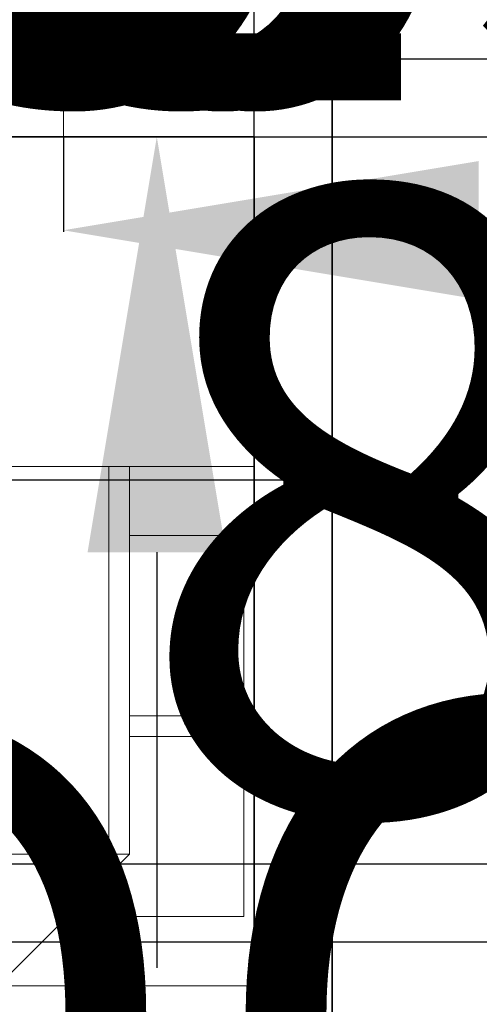
# Model space of a CAD drawing. Units: inches. Extents: x -307 to 2141, y -58 to 895.
# Tile 24 of 28: x 880 to 933, y 582 to 696. Entities that reach past the tile are written whole.
import ezdxf

# ---------------------------------------------------------------- set-up
doc = ezdxf.new("R2010")
doc.units = ezdxf.units.IN
doc.header["$MEASUREMENT"] = 0
for name, color, linetype, lineweight in [('A-ANNO-DIMS', 2, 'Continuous', 18), ('A-FURN', 8, 'Continuous', 18), ('A-GLAZ', 4, 'Continuous', 18), ('A-WALL', 7, 'Continuous', 35)]:
    doc.layers.add(name, color=color, linetype=linetype, lineweight=lineweight)
doc.styles.get("Standard").update_dxf_attribs({"font": 'arial.ttf'})
doc.dimstyles.get("Standard").update_dxf_attribs({"dimtxt": 72, "dimasz": 48, "dimexe": 0.18, "dimexo": 0.0625, "dimgap": 0.09, "dimtad": 0, "dimtih": 1, "dimtoh": 1, "dimdec": 0, "dimrnd": 48, "dimzin": 0, "dimdsep": 46, "dimlunit": 3, "dimtxsty": 'Standard', "dimcen": 0.09, "dimadec": 0, "dimazin": 0, "dimtfac": 1, "dimtdec": 0, "dimtofl": 0, "dimtmove": 0, "dimatfit": 3, "dimfxl": 1, "dimtolj": 1, "dimtzin": 0, "dimarcsym": 0})

# ---------------------------------------------------------------- blocks, each defined once
blk = doc.blocks.new('Bed - Queen')
for p, q in [((0, -80.00003), (0, 0)), ((0, 0), (59.99999, 0)), ((59.99999, 0), (59.99999, -80.00003)), ((7.99999, -1.2), (28.79998, -1.2)), ((7.99999, -14.4), (7.99999, -1.2)), ((28.79998, -1.2), (28.79998, -14.4)), ((31.19999, -1.2), (51.99999, -1.2)), ((31.19999, -14.4), (31.19999, -1.2)), ((51.99999, -1.2), (51.99999, -16.4)), ((0, -14.4), (44.8, -14.4)), ((59.99999, -29.6), (44.8, -14.4)), ((44.8, -14.4), (44.8, -29.6)), ((44.8, -16.8), (0, -16.8)), ((51.99999, -16.4), (46.79936, -16.4)), ((44.8, -29.6), (59.99999, -29.6)), ((59.99999, -80.00003), (0, -80.00003))]:
    blk.add_line(p, q)
blk = doc.blocks.new('WIN-72IN')
blk.add_line((72, 4.5), (0, 4.5))
blk.add_lwpolyline([(72, 0), (0, 0), (0, 9), (72, 9)], close=True)
blk = doc.blocks.new('*D30')
at = {"layer": 'A-ANNO-DIMS', "color": 0, "lineweight": -2, "transparency": 16777216}
for p, q in [((570.74, 532.83), (570.74, 580.83)), ((570.74, 580.83), (618.74, 580.83)), ((565.4, 484.83), (570.92, 484.83)), ((565.4, 448.83), (570.92, 448.83)), ((570.74, 400.83), (570.74, 352.83))]:
    blk.add_line(p, q, dxfattribs=at)
at = {"layer": 'A-ANNO-DIMS', "color": 0, "transparency": 16777216}
for points in [[(562.74, 532.83), (578.74, 532.83), (570.74, 484.83)], [(562.74, 400.83), (578.74, 400.83), (570.74, 448.83)]]:
    blk.add_solid(points, dxfattribs=at)
at = {"layer": 'Defpoints', "color": 0, "transparency": 16777216}
for p in [(565.34, 484.83), (570.74, 484.83), (565.34, 448.83)]:
    blk.add_point(p, dxfattribs=at)
at = {"layer": 'A-ANNO-DIMS', "color": 0, "transparency": 16777216, "insert": (1030.17, 580.83), "char_height": 72, "attachment_point": 5}
blk.add_mtext('\\A1;WINDOW 36 TYP.', dxfattribs=at)
blk = doc.blocks.new('*D32')
at = {"layer": 'A-ANNO-DIMS', "color": 0, "lineweight": -2, "transparency": 16777216}
for p, q in [((813.29, 682.28), (813.29, 671.36)), ((885.29, 682.28), (885.29, 671.36)), ((765.29, 671.54), (717.29, 671.54)), ((933.29, 671.54), (981.29, 671.54))]:
    blk.add_line(p, q, dxfattribs=at)
at = {"layer": 'A-ANNO-DIMS', "color": 0, "transparency": 16777216}
for points in [[(765.29, 679.54), (765.29, 663.54), (813.29, 671.54)], [(933.29, 679.54), (933.29, 663.54), (885.29, 671.54)]]:
    blk.add_solid(points, dxfattribs=at)
at = {"layer": 'Defpoints', "color": 0, "transparency": 16777216}
for p in [(813.29, 682.34), (885.29, 682.34), (885.29, 671.54)]:
    blk.add_point(p, dxfattribs=at)
at = {"layer": 'A-ANNO-DIMS', "color": 0, "transparency": 16777216, "insert": (1392.73, 671.54), "char_height": 72, "attachment_point": 5}
blk.add_mtext('\\A1;WINDOW 72 TYP.', dxfattribs=at)
blk = doc.blocks.new('*D33')
at = {"layer": 'A-ANNO-DIMS', "color": 0, "lineweight": -2, "transparency": 16777216}
for p, q in [((896.09, 739.34), (896.09, 787.34)), ((896.09, 787.34), (944.09, 787.34)), ((885.36, 691.34), (896.27, 691.34)), ((885.36, 682.34), (896.27, 682.34)), ((896.09, 634.34), (896.09, 586.34))]:
    blk.add_line(p, q, dxfattribs=at)
at = {"layer": 'A-ANNO-DIMS', "color": 0, "transparency": 16777216}
for points in [[(888.09, 739.34), (904.09, 739.34), (896.09, 691.34)], [(888.09, 634.34), (904.09, 634.34), (896.09, 682.34)]]:
    blk.add_solid(points, dxfattribs=at)
at = {"layer": 'Defpoints', "color": 0, "transparency": 16777216}
for p in [(885.29, 691.34), (896.09, 691.34), (885.29, 682.34)]:
    blk.add_point(p, dxfattribs=at)
at = {"layer": 'A-ANNO-DIMS', "color": 0, "transparency": 16777216, "insert": (1091.45, 787.34), "char_height": 72, "attachment_point": 5}
blk.add_mtext('\\A1;9 TYP.', dxfattribs=at)
blk = doc.blocks.new('*D34')
at = {"layer": 'A-ANNO-DIMS', "color": 0, "lineweight": -2, "transparency": 16777216}
for p, q in [((927.14, 490.97), (927.14, 538.97)), ((927.14, 538.97), (975.14, 538.97)), ((916.4, 442.97), (927.32, 442.97)), ((916.4, 370.95), (927.32, 370.95)), ((927.14, 322.95), (927.14, 274.95))]:
    blk.add_line(p, q, dxfattribs=at)
at = {"layer": 'A-ANNO-DIMS', "color": 0, "transparency": 16777216}
for points in [[(919.14, 490.97), (935.14, 490.97), (927.14, 442.97)], [(919.14, 322.95), (935.14, 322.95), (927.14, 370.95)]]:
    blk.add_solid(points, dxfattribs=at)
at = {"layer": 'Defpoints', "color": 0, "transparency": 16777216}
for p in [(916.34, 442.97), (927.14, 442.97), (916.34, 370.95)]:
    blk.add_point(p, dxfattribs=at)
at = {"layer": 'A-ANNO-DIMS', "color": 0, "transparency": 16777216, "insert": (1584.53, 538.97), "char_height": 72, "attachment_point": 5}
blk.add_mtext('\\A1;PAIRED WINDOW 72 TYP.', dxfattribs=at)
blk = doc.blocks.new('*D37')
at = {"layer": 'A-ANNO-DIMS', "color": 0, "lineweight": -2, "transparency": 16777216}
for p, q in [((828.62, 519.41), (780.62, 519.46)), ((876.61, 514.46), (876.62, 519.54)), ((897.61, 514.44), (897.62, 519.51)), ((945.62, 519.28), (993.62, 519.22))]:
    blk.add_line(p, q, dxfattribs=at)
at = {"layer": 'A-ANNO-DIMS', "color": 0, "transparency": 16777216}
for points in [[(828.63, 527.41), (828.61, 511.41), (876.62, 519.36)], [(945.63, 527.28), (945.61, 511.28), (897.62, 519.33)]]:
    blk.add_solid(points, dxfattribs=at)
at = {"layer": 'Defpoints', "color": 0, "transparency": 16777216}
for p in [(876.62, 519.36), (876.61, 514.4), (897.61, 514.38)]:
    blk.add_point(p, dxfattribs=at)
at = {"layer": 'A-ANNO-DIMS', "color": 0, "transparency": 16777216, "insert": (604.68, 519.46), "char_height": 72, "attachment_point": 5}
blk.add_mtext('\\A1;21 TYP.', dxfattribs=at)
blk = doc.blocks.new('*D42')
at = {"layer": 'A-ANNO-DIMS', "color": 0, "lineweight": -2, "transparency": 16777216}
for p, q in [((880.26, 543.86), (928.25, 544.87)), ((822.3, 541.2), (822.27, 542.82)), ((832.3, 541.41), (832.27, 543.03)), ((774.28, 541.63), (726.29, 540.62))]:
    blk.add_line(p, q, dxfattribs=at)
at = {"layer": 'A-ANNO-DIMS', "color": 0, "transparency": 16777216}
for points in [[(880.09, 551.86), (880.43, 535.86), (832.27, 542.85)], [(774.11, 549.63), (774.45, 533.63), (822.27, 542.64)]]:
    blk.add_solid(points, dxfattribs=at)
at = {"layer": 'Defpoints', "color": 0, "transparency": 16777216}
for p in [(832.27, 542.85), (822.3, 541.14), (832.3, 541.35)]:
    blk.add_point(p, dxfattribs=at)
at = {"layer": 'A-ANNO-DIMS', "color": 0, "transparency": 16777216, "insert": (1192.89, 544.87), "char_height": 72, "attachment_point": 5}
blk.add_mtext('\\A1;FAUCET 10', dxfattribs=at)
blk = doc.blocks.new('*D44')
at = {"layer": 'A-ANNO-DIMS', "color": 0, "lineweight": -2, "transparency": 16777216}
for p, q in [((839.87, 521.22), (839.95, 517.42)), ((815.33, 520.71), (815.41, 516.91)), ((887.94, 518.61), (935.93, 519.62)), ((767.41, 516.08), (719.42, 515.07))]:
    blk.add_line(p, q, dxfattribs=at)
at = {"layer": 'A-ANNO-DIMS', "color": 0, "transparency": 16777216}
for points in [[(887.77, 526.61), (888.11, 510.61), (839.95, 517.6)], [(767.25, 524.08), (767.58, 508.08), (815.4, 517.09)]]:
    blk.add_solid(points, dxfattribs=at)
at = {"layer": 'Defpoints', "color": 0, "transparency": 16777216}
for p in [(839.87, 521.29), (815.33, 520.77), (839.95, 517.6)]:
    blk.add_point(p, dxfattribs=at)
at = {"layer": 'A-ANNO-DIMS', "color": 0, "transparency": 16777216, "insert": (1151.16, 519.62), "char_height": 72, "attachment_point": 5}
blk.add_mtext('\\A1;BASIN 25', dxfattribs=at)
blk = doc.blocks.new('*D46')
at = {"layer": 'A-ANNO-DIMS', "color": 0, "lineweight": -2, "transparency": 16777216}
for p, q in [((801.41, 645.78), (801.41, 642.52)), ((822.41, 645.78), (822.41, 642.52)), ((753.41, 642.7), (705.41, 642.7)), ((870.41, 642.7), (918.41, 642.7))]:
    blk.add_line(p, q, dxfattribs=at)
at = {"layer": 'A-ANNO-DIMS', "color": 0, "transparency": 16777216}
for points in [[(753.41, 650.7), (753.41, 634.7), (801.41, 642.7)], [(870.41, 650.7), (870.41, 634.7), (822.41, 642.7)]]:
    blk.add_solid(points, dxfattribs=at)
at = {"layer": 'Defpoints', "color": 0, "transparency": 16777216}
for p in [(801.41, 645.85), (822.41, 645.85), (822.41, 642.7)]:
    blk.add_point(p, dxfattribs=at)
at = {"layer": 'A-ANNO-DIMS', "color": 0, "transparency": 16777216, "insert": (1282.7, 642.7), "char_height": 72, "attachment_point": 5}
blk.add_mtext('\\A1;DESK CHAIR 21', dxfattribs=at)
blk = doc.blocks.new('*D47')
at = {"layer": 'A-ANNO-DIMS', "color": 0, "lineweight": -2, "transparency": 16777216}
for p, q in [((825.56, 711.18), (825.56, 759.18)), ((825.56, 759.18), (873.56, 759.18)), ((822.48, 663.18), (825.74, 663.18)), ((822.48, 645.85), (825.74, 645.85)), ((825.56, 597.85), (825.56, 549.85))]:
    blk.add_line(p, q, dxfattribs=at)
at = {"layer": 'A-ANNO-DIMS', "color": 0, "transparency": 16777216}
for points in [[(817.56, 711.18), (833.56, 711.18), (825.56, 663.18)], [(817.56, 597.85), (833.56, 597.85), (825.56, 645.85)]]:
    blk.add_solid(points, dxfattribs=at)
at = {"layer": 'Defpoints', "color": 0, "transparency": 16777216}
for p in [(822.41, 663.18), (825.56, 663.18), (822.41, 645.85)]:
    blk.add_point(p, dxfattribs=at)
at = {"layer": 'A-ANNO-DIMS', "color": 0, "transparency": 16777216, "insert": (921.83, 759.18), "char_height": 72, "attachment_point": 5}
blk.add_mtext('\\A1;17', dxfattribs=at)
blk = doc.blocks.new('*D52')
at = {"layer": 'A-ANNO-DIMS', "color": 0, "lineweight": -2, "transparency": 16777216}
for p, q in [((660.21, 554.25), (660.21, 602.25)), ((673.8, 506.25), (660.03, 506.25)), ((673.8, 415.25), (660.03, 415.25)), ((660.21, 367.25), (660.21, 319.25))]:
    blk.add_line(p, q, dxfattribs=at)
at = {"layer": 'A-ANNO-DIMS', "color": 0, "transparency": 16777216}
for points in [[(652.21, 554.25), (668.21, 554.25), (660.21, 506.25)], [(652.21, 367.25), (668.21, 367.25), (660.21, 415.25)]]:
    blk.add_solid(points, dxfattribs=at)
at = {"layer": 'Defpoints', "color": 0, "transparency": 16777216}
for p in [(673.86, 506.25), (660.21, 415.25), (673.86, 415.25)]:
    blk.add_point(p, dxfattribs=at)
at = {"layer": 'A-ANNO-DIMS', "color": 0, "transparency": 16777216, "insert": (660.21, 460.75), "char_height": 72, "attachment_point": 5}
blk.add_mtext('\\A1;DINING SET 91', dxfattribs=at)
blk = doc.blocks.new('*D56')
at = {"layer": 'A-ANNO-DIMS', "color": 0, "lineweight": -2, "transparency": 16777216}
for p, q in [((679.73, 723.21), (679.73, 771.21)), ((679.73, 771.21), (727.73, 771.21)), ((675.74, 675.21), (679.91, 675.21)), ((675.74, 648.21), (679.91, 648.21)), ((679.73, 600.21), (679.73, 552.21))]:
    blk.add_line(p, q, dxfattribs=at)
at = {"layer": 'A-ANNO-DIMS', "color": 0, "transparency": 16777216}
for points in [[(671.73, 723.21), (687.73, 723.21), (679.73, 675.21)], [(671.73, 600.21), (687.73, 600.21), (679.73, 648.21)]]:
    blk.add_solid(points, dxfattribs=at)
at = {"layer": 'Defpoints', "color": 0, "transparency": 16777216}
for p in [(675.68, 675.21), (679.73, 675.21), (675.68, 648.21)]:
    blk.add_point(p, dxfattribs=at)
at = {"layer": 'A-ANNO-DIMS', "color": 0, "transparency": 16777216, "insert": (1006.66, 771.21), "char_height": 72, "attachment_point": 5}
blk.add_mtext('\\A1;ROCKER 27', dxfattribs=at)
blk = doc.blocks.new('*D62')
at = {"layer": 'A-ANNO-DIMS', "color": 0, "lineweight": -2, "transparency": 16777216}
for p, q in [((556.34, 691.4), (556.34, 722.72)), ((604.34, 722.54), (656.85, 722.54)), ((868.34, 722.54), (815.82, 722.54)), ((916.34, 490.97), (916.34, 722.72))]:
    blk.add_line(p, q, dxfattribs=at)
at = {"layer": 'A-ANNO-DIMS', "color": 0, "transparency": 16777216}
for points in [[(604.34, 730.54), (604.34, 714.54), (556.34, 722.54)], [(868.34, 730.54), (868.34, 714.54), (916.34, 722.54)]]:
    blk.add_solid(points, dxfattribs=at)
at = {"layer": 'Defpoints', "color": 0, "transparency": 16777216}
for p in [(916.34, 722.54), (556.34, 691.34), (916.34, 490.9)]:
    blk.add_point(p, dxfattribs=at)
at = {"layer": 'A-ANNO-DIMS', "color": 0, "transparency": 16777216, "insert": (736.34, 722.54), "char_height": 72, "attachment_point": 5}
blk.add_mtext('\\A1;360', dxfattribs=at)
blk = doc.blocks.new('*D63')
at = {"layer": 'A-ANNO-DIMS', "color": 0, "lineweight": -2, "transparency": 16777216}
for p, q in [((916.4, 691.34), (947.72, 691.34)), ((947.54, 643.34), (947.54, 416.19)), ((947.54, 115.34), (947.54, 342.49)), ((704.68, 67.34), (947.72, 67.34))]:
    blk.add_line(p, q, dxfattribs=at)
at = {"layer": 'A-ANNO-DIMS', "color": 0, "transparency": 16777216}
for points in [[(939.54, 643.34), (955.54, 643.34), (947.54, 691.34)], [(939.54, 115.34), (955.54, 115.34), (947.54, 67.34)]]:
    blk.add_solid(points, dxfattribs=at)
at = {"layer": 'Defpoints', "color": 0, "transparency": 16777216}
for p in [(916.34, 691.34), (704.62, 67.34), (947.54, 67.34)]:
    blk.add_point(p, dxfattribs=at)
at = {"layer": 'A-ANNO-DIMS', "color": 0, "transparency": 16777216, "insert": (947.54, 379.34), "char_height": 72, "attachment_point": 5}
blk.add_mtext('\\A1;624', dxfattribs=at)
blk = doc.blocks.new('*D75')
at = {"layer": 'A-ANNO-DIMS', "color": 0, "lineweight": -2, "transparency": 16777216}
for p, q in [((565.34, 682.4), (565.34, 722.72)), ((613.34, 722.54), (637.34, 722.54)), ((685.34, 682.4), (685.34, 722.72)), ((685.34, 722.54), (733.34, 722.54))]:
    blk.add_line(p, q, dxfattribs=at)
at = {"layer": 'A-ANNO-DIMS', "color": 0, "transparency": 16777216}
for points in [[(613.34, 730.54), (613.34, 714.54), (565.34, 722.54)], [(637.34, 730.54), (637.34, 714.54), (685.34, 722.54)]]:
    blk.add_solid(points, dxfattribs=at)
at = {"layer": 'Defpoints', "color": 0, "transparency": 16777216}
for p in [(685.34, 722.54), (565.34, 682.34), (685.34, 682.34)]:
    blk.add_point(p, dxfattribs=at)
at = {"layer": 'A-ANNO-DIMS', "color": 0, "transparency": 16777216, "insert": (809.45, 722.54), "char_height": 72, "attachment_point": 5}
blk.add_mtext('\\A1;120', dxfattribs=at)
blk = doc.blocks.new('*D76')
at = {"layer": 'A-ANNO-DIMS', "color": 0, "lineweight": -2, "transparency": 16777216}
for p, q in [((646.34, 722.54), (598.34, 722.54)), ((694.34, 682.4), (694.34, 722.72)), ((778.34, 682.4), (778.34, 722.72)), ((826.34, 722.54), (874.34, 722.54))]:
    blk.add_line(p, q, dxfattribs=at)
at = {"layer": 'A-ANNO-DIMS', "color": 0, "transparency": 16777216}
for points in [[(646.34, 730.54), (646.34, 714.54), (694.34, 722.54)], [(826.34, 730.54), (826.34, 714.54), (778.34, 722.54)]]:
    blk.add_solid(points, dxfattribs=at)
at = {"layer": 'Defpoints', "color": 0, "transparency": 16777216}
for p in [(778.34, 722.54), (694.34, 682.34), (778.34, 682.34)]:
    blk.add_point(p, dxfattribs=at)
at = {"layer": 'A-ANNO-DIMS', "color": 0, "transparency": 16777216, "insert": (925.9, 722.54), "char_height": 72, "attachment_point": 5}
blk.add_mtext('\\A1;84', dxfattribs=at)
blk = doc.blocks.new('*D77')
at = {"layer": 'A-ANNO-DIMS', "color": 0, "lineweight": -2, "transparency": 16777216}
for p, q in [((787.34, 682.4), (787.34, 722.72)), ((835.34, 722.54), (859.34, 722.54)), ((907.34, 682.4), (907.34, 722.72)), ((907.34, 722.54), (955.34, 722.54))]:
    blk.add_line(p, q, dxfattribs=at)
at = {"layer": 'A-ANNO-DIMS', "color": 0, "transparency": 16777216}
for points in [[(835.34, 730.54), (835.34, 714.54), (787.34, 722.54)], [(859.34, 730.54), (859.34, 714.54), (907.34, 722.54)]]:
    blk.add_solid(points, dxfattribs=at)
at = {"layer": 'Defpoints', "color": 0, "transparency": 16777216}
for p in [(907.34, 722.54), (787.34, 682.34), (907.34, 682.34)]:
    blk.add_point(p, dxfattribs=at)
at = {"layer": 'A-ANNO-DIMS', "color": 0, "transparency": 16777216, "insert": (1031.45, 722.54), "char_height": 72, "attachment_point": 5}
blk.add_mtext('\\A1;120', dxfattribs=at)
blk = doc.blocks.new('*D78')
at = {"layer": 'A-ANNO-DIMS', "color": 0, "lineweight": -2, "transparency": 16777216}
for p, q in [((947.53984, 730.340828), (947.53984, 778.340828)), ((778.39834, 682.340828), (947.71984, 682.340828)), ((730.39834, 598.340828), (947.71984, 598.340828)), ((947.53984, 550.340828), (947.53984, 502.340828))]:
    blk.add_line(p, q, dxfattribs=at)
at = {"layer": 'A-ANNO-DIMS', "color": 0, "transparency": 16777216}
for points in [[(939.53984, 730.340828), (955.53984, 730.340828), (947.53984, 682.340828)], [(939.53984, 550.340828), (955.53984, 550.340828), (947.53984, 598.340828)]]:
    blk.add_solid(points, dxfattribs=at)
at = {"layer": 'Defpoints', "color": 0, "transparency": 16777216}
for p in [(778.33584, 682.340828), (947.53984, 682.340828), (730.33584, 598.340828)]:
    blk.add_point(p, dxfattribs=at)
at = {"layer": 'A-ANNO-DIMS', "color": 0, "transparency": 16777216, "insert": (947.53984, 640.340828), "char_height": 72, "attachment_point": 5}
blk.add_mtext('\\A1;84', dxfattribs=at)
blk = doc.blocks.new('*D79')
at = {"layer": 'A-ANNO-DIMS', "color": 0, "lineweight": -2, "transparency": 16777216}
for p, q in [((947.54, 682.34), (947.54, 730.34)), ((947.54, 730.34), (995.54, 730.34)), ((907.4, 682.34), (947.72, 682.34)), ((947.54, 598.34), (947.54, 634.34)), ((907.4, 550.34), (947.72, 550.34))]:
    blk.add_line(p, q, dxfattribs=at)
at = {"layer": 'A-ANNO-DIMS', "color": 0, "transparency": 16777216}
for points in [[(939.54, 634.34), (955.54, 634.34), (947.54, 682.34)], [(939.54, 598.34), (955.54, 598.34), (947.54, 550.34)]]:
    blk.add_solid(points, dxfattribs=at)
at = {"layer": 'Defpoints', "color": 0, "transparency": 16777216}
for p in [(907.34, 682.34), (947.54, 682.34), (907.34, 550.34)]:
    blk.add_point(p, dxfattribs=at)
at = {"layer": 'A-ANNO-DIMS', "color": 0, "transparency": 16777216, "insert": (1071.41, 730.34), "char_height": 72, "attachment_point": 5}
blk.add_mtext('\\A1;132', dxfattribs=at)
blk = doc.blocks.new('*D80')
at = {"layer": 'A-ANNO-DIMS', "color": 0, "lineweight": -2, "transparency": 16777216}
for p, q in [((763.34, 722.54), (715.34, 722.54)), ((811.34, 517.4), (811.34, 722.72)), ((907.34, 541.4), (907.34, 722.72)), ((955.34, 722.54), (1003.34, 722.54))]:
    blk.add_line(p, q, dxfattribs=at)
at = {"layer": 'A-ANNO-DIMS', "color": 0, "transparency": 16777216}
for points in [[(763.34, 730.54), (763.34, 714.54), (811.34, 722.54)], [(955.34, 730.54), (955.34, 714.54), (907.34, 722.54)]]:
    blk.add_solid(points, dxfattribs=at)
at = {"layer": 'Defpoints', "color": 0, "transparency": 16777216}
for p in [(907.34, 722.54), (907.34, 541.34), (811.34, 517.34)]:
    blk.add_point(p, dxfattribs=at)
at = {"layer": 'A-ANNO-DIMS', "color": 0, "transparency": 16777216, "insert": (1054.97, 722.54), "char_height": 72, "attachment_point": 5}
blk.add_mtext('\\A1;96', dxfattribs=at)
blk = doc.blocks.new('*D81')
at = {"layer": 'A-ANNO-DIMS', "color": 0, "lineweight": -2, "transparency": 16777216}
for p, q in [((947.54, 589.34), (947.54, 637.34)), ((947.54, 637.34), (995.54, 637.34)), ((907.4, 541.34), (947.72, 541.34)), ((907.4, 481.34), (947.72, 481.34)), ((947.54, 433.34), (947.54, 385.34))]:
    blk.add_line(p, q, dxfattribs=at)
at = {"layer": 'A-ANNO-DIMS', "color": 0, "transparency": 16777216}
for points in [[(939.54, 589.34), (955.54, 589.34), (947.54, 541.34)], [(939.54, 433.34), (955.54, 433.34), (947.54, 481.34)]]:
    blk.add_solid(points, dxfattribs=at)
at = {"layer": 'Defpoints', "color": 0, "transparency": 16777216}
for p in [(907.34, 541.34), (947.54, 541.34), (907.34, 481.34)]:
    blk.add_point(p, dxfattribs=at)
at = {"layer": 'A-ANNO-DIMS', "color": 0, "transparency": 16777216, "insert": (1047.27, 637.34), "char_height": 72, "attachment_point": 5}
blk.add_mtext('\\A1;60', dxfattribs=at)
blk = doc.blocks.new('*D83')
at = {"layer": 'A-ANNO-DIMS', "color": 0, "lineweight": -2, "transparency": 16777216}
for p, q in [((947.54, 538.9), (947.54, 586.9)), ((916.4, 490.9), (947.72, 490.9)), ((907.4, 481.34), (947.72, 481.34)), ((947.54, 433.34), (947.54, 385.34)), ((947.54, 385.34), (899.54, 385.34))]:
    blk.add_line(p, q, dxfattribs=at)
at = {"layer": 'A-ANNO-DIMS', "color": 0, "transparency": 16777216}
for points in [[(939.54, 538.9), (955.54, 538.9), (947.54, 490.9)], [(939.54, 433.34), (955.54, 433.34), (947.54, 481.34)]]:
    blk.add_solid(points, dxfattribs=at)
at = {"layer": 'Defpoints', "color": 0, "transparency": 16777216}
for p in [(916.34, 490.9), (907.34, 481.34), (947.54, 481.34)]:
    blk.add_point(p, dxfattribs=at)
at = {"layer": 'A-ANNO-DIMS', "color": 0, "transparency": 16777216, "insert": (777.97, 385.34), "char_height": 72, "attachment_point": 5}
blk.add_mtext('\\A1;9.563', dxfattribs=at)
blk = doc.blocks.new('*D94')
at = {"layer": 'A-ANNO-DIMS', "color": 0, "lineweight": -2, "transparency": 16777216}
for p, q in [((517.34, 722.54), (469.34, 722.54)), ((565.34, 529.4), (565.34, 722.72)), ((629.84, 529.4), (629.84, 722.72)), ((677.84, 722.54), (725.84, 722.54))]:
    blk.add_line(p, q, dxfattribs=at)
at = {"layer": 'A-ANNO-DIMS', "color": 0, "transparency": 16777216}
for points in [[(517.34, 730.54), (517.34, 714.54), (565.34, 722.54)], [(677.84, 730.54), (677.84, 714.54), (629.84, 722.54)]]:
    blk.add_solid(points, dxfattribs=at)
at = {"layer": 'Defpoints', "color": 0, "transparency": 16777216}
for p in [(629.84, 722.54), (565.34, 529.34), (629.84, 529.34)]:
    blk.add_point(p, dxfattribs=at)
at = {"layer": 'A-ANNO-DIMS', "color": 0, "transparency": 16777216, "insert": (819.9, 722.54), "char_height": 72, "attachment_point": 5}
blk.add_mtext('\\A1;64.5', dxfattribs=at)
blk = doc.blocks.new('*D95')
at = {"layer": 'A-ANNO-DIMS', "color": 0, "lineweight": -2, "transparency": 16777216}
for p, q in [((947.54, 577.34), (947.54, 625.34)), ((947.54, 625.34), (995.54, 625.34)), ((629.9, 529.34), (947.72, 529.34)), ((629.9, 502.66), (947.72, 502.66)), ((947.54, 454.66), (947.54, 406.66))]:
    blk.add_line(p, q, dxfattribs=at)
at = {"layer": 'A-ANNO-DIMS', "color": 0, "transparency": 16777216}
for points in [[(939.54, 577.34), (955.54, 577.34), (947.54, 529.34)], [(939.54, 454.66), (955.54, 454.66), (947.54, 502.66)]]:
    blk.add_solid(points, dxfattribs=at)
at = {"layer": 'Defpoints', "color": 0, "transparency": 16777216}
for p in [(629.84, 529.34), (947.54, 529.34), (629.84, 502.66)]:
    blk.add_point(p, dxfattribs=at)
at = {"layer": 'A-ANNO-DIMS', "color": 0, "transparency": 16777216, "insert": (1117.8, 625.34), "char_height": 72, "attachment_point": 5}
blk.add_mtext('\\A1;26.68', dxfattribs=at)
blk = doc.blocks.new('*D96')
at = {"layer": 'A-ANNO-DIMS', "color": 0, "lineweight": -2, "transparency": 16777216}
for p, q in [((646.34, 722.54), (598.34, 722.54)), ((694.34, 598.4), (694.34, 722.72)), ((730.34, 598.4), (730.34, 722.72)), ((778.34, 722.54), (826.34, 722.54))]:
    blk.add_line(p, q, dxfattribs=at)
at = {"layer": 'A-ANNO-DIMS', "color": 0, "transparency": 16777216}
for points in [[(646.34, 730.54), (646.34, 714.54), (694.34, 722.54)], [(778.34, 730.54), (778.34, 714.54), (730.34, 722.54)]]:
    blk.add_solid(points, dxfattribs=at)
at = {"layer": 'Defpoints', "color": 0, "transparency": 16777216}
for p in [(730.34, 722.54), (694.34, 598.34), (730.34, 598.34)]:
    blk.add_point(p, dxfattribs=at)
at = {"layer": 'A-ANNO-DIMS', "color": 0, "transparency": 16777216, "insert": (877.95, 722.54), "char_height": 72, "attachment_point": 5}
blk.add_mtext('\\A1;36', dxfattribs=at)
blk = doc.blocks.new('*D97')
at = {"layer": 'A-ANNO-DIMS', "color": 0, "lineweight": -2, "transparency": 16777216}
for p, q in [((947.54, 637.34), (947.54, 685.34)), ((947.54, 685.34), (995.54, 685.34)), ((685.4, 589.34), (947.72, 589.34)), ((685.4, 538.34), (947.72, 538.34)), ((947.54, 490.34), (947.54, 442.34))]:
    blk.add_line(p, q, dxfattribs=at)
at = {"layer": 'A-ANNO-DIMS', "color": 0, "transparency": 16777216}
for points in [[(939.54, 637.34), (955.54, 637.34), (947.54, 589.34)], [(939.54, 490.34), (955.54, 490.34), (947.54, 538.34)]]:
    blk.add_solid(points, dxfattribs=at)
at = {"layer": 'Defpoints', "color": 0, "transparency": 16777216}
for p in [(685.34, 589.34), (947.54, 589.34), (685.34, 538.34)]:
    blk.add_point(p, dxfattribs=at)
at = {"layer": 'A-ANNO-DIMS', "color": 0, "transparency": 16777216, "insert": (1040.25, 685.34), "char_height": 72, "attachment_point": 5}
blk.add_mtext('\\A1;51', dxfattribs=at)
blk = doc.blocks.new('*D101')
at = {"layer": 'A-ANNO-DIMS', "color": 0, "lineweight": -2, "transparency": 16777216}
for p, q in [((508.34, 722.54), (460.34, 722.54)), ((556.34, 691.4), (556.34, 722.72)), ((589.36, 691.4), (589.36, 722.72)), ((637.36, 722.54), (685.36, 722.54))]:
    blk.add_line(p, q, dxfattribs=at)
at = {"layer": 'A-ANNO-DIMS', "color": 0, "transparency": 16777216}
for points in [[(508.34, 730.54), (508.34, 714.54), (556.34, 722.54)], [(637.36, 730.54), (637.36, 714.54), (589.36, 722.54)]]:
    blk.add_solid(points, dxfattribs=at)
at = {"layer": 'Defpoints', "color": 0, "transparency": 16777216}
for p in [(589.36, 722.54), (556.34, 691.34), (589.36, 691.34)]:
    blk.add_point(p, dxfattribs=at)
at = {"layer": 'A-ANNO-DIMS', "color": 0, "transparency": 16777216, "insert": (806.54, 722.54), "char_height": 72, "attachment_point": 5}
blk.add_mtext('\\A1;33.02', dxfattribs=at)
blk = doc.blocks.new('*D102')
at = {"layer": 'A-ANNO-DIMS', "color": 0, "lineweight": -2, "transparency": 16777216}
for p, q in [((837.29, 722.54), (789.29, 722.54)), ((885.29, 691.4), (885.29, 722.72)), ((916.34, 691.4), (916.34, 722.72)), ((964.34, 722.54), (1012.34, 722.54))]:
    blk.add_line(p, q, dxfattribs=at)
at = {"layer": 'A-ANNO-DIMS', "color": 0, "transparency": 16777216}
for points in [[(837.29, 730.54), (837.29, 714.54), (885.29, 722.54)], [(964.34, 730.54), (964.34, 714.54), (916.34, 722.54)]]:
    blk.add_solid(points, dxfattribs=at)
at = {"layer": 'Defpoints', "color": 0, "transparency": 16777216}
for p in [(916.34, 722.54), (885.29, 691.34), (916.34, 691.34)]:
    blk.add_point(p, dxfattribs=at)
at = {"layer": 'A-ANNO-DIMS', "color": 0, "transparency": 16777216, "insert": (1133.74, 722.54), "char_height": 72, "attachment_point": 5}
blk.add_mtext('\\A1;31.04', dxfattribs=at)
blk = doc.blocks.new('*D107')
at = {"layer": 'A-ANNO-DIMS', "color": 0, "lineweight": -2, "transparency": 16777216}
for p, q in [((517.34, 722.54), (469.34, 722.54)), ((565.34, 409.4), (565.34, 722.72)), ((589.34, 409.4), (589.34, 722.72)), ((637.34, 722.54), (685.34, 722.54))]:
    blk.add_line(p, q, dxfattribs=at)
at = {"layer": 'A-ANNO-DIMS', "color": 0, "transparency": 16777216}
for points in [[(517.34, 730.54), (517.34, 714.54), (565.34, 722.54)], [(637.34, 730.54), (637.34, 714.54), (589.34, 722.54)]]:
    blk.add_solid(points, dxfattribs=at)
at = {"layer": 'Defpoints', "color": 0, "transparency": 16777216}
for p in [(589.34, 722.54), (565.34, 409.34), (589.34, 409.34)]:
    blk.add_point(p, dxfattribs=at)
at = {"layer": 'A-ANNO-DIMS', "color": 0, "transparency": 16777216, "insert": (835.49, 722.54), "char_height": 72, "attachment_point": 5}
blk.add_mtext('\\A1;24.003', dxfattribs=at)
blk = doc.blocks.new('*D108')
at = {"layer": 'A-ANNO-DIMS', "color": 0, "lineweight": -2, "transparency": 16777216}
for p, q in [((947.54, 550.66), (947.54, 598.66)), ((589.4, 502.66), (947.72, 502.66)), ((589.4, 409.34), (947.72, 409.34)), ((947.54, 361.34), (947.54, 313.34))]:
    blk.add_line(p, q, dxfattribs=at)
at = {"layer": 'A-ANNO-DIMS', "color": 0, "transparency": 16777216}
for points in [[(939.54, 550.66), (955.54, 550.66), (947.54, 502.66)], [(939.54, 361.34), (955.54, 361.34), (947.54, 409.34)]]:
    blk.add_solid(points, dxfattribs=at)
at = {"layer": 'Defpoints', "color": 0, "transparency": 16777216}
for p in [(589.34, 502.66), (947.54, 502.66), (589.34, 409.34)]:
    blk.add_point(p, dxfattribs=at)
at = {"layer": 'A-ANNO-DIMS', "color": 0, "transparency": 16777216, "insert": (947.54, 456), "char_height": 72, "attachment_point": 5}
blk.add_mtext('\\A1;93.32', dxfattribs=at)

msp = doc.modelspace()

# ---------------------------------------------------------------- linework, layer by layer
at = {"layer": 'A-WALL'}
for p, q in [((916.3358, 691.3408), (556.3358, 691.3408)), ((916.3358, 166.3408), (916.3358, 691.3408)), ((907.3358, 682.3408), (565.3358, 682.3408)), ((907.3358, 166.3408), (907.3358, 682.3408))]:
    msp.add_line(p, q, dxfattribs=at)

# ---------------------------------------------------------------- block references
at = {"layer": 'A-FURN', "rotation": 270}
msp.add_blockref('Bed - Queen', (907.3358, 644.2648), dxfattribs=at)
at = {"layer": 'A-GLAZ'}
msp.add_blockref('WIN-72IN', (813.293, 682.341), dxfattribs=at)

# ---------------------------------------------------------------- dimensions: what is measured, and where the dimension line sits
at = {"layer": 'A-ANNO-DIMS'}
for base, p1, p2, angle, text, picture, middle in [((896.0934, 691.3408), (885.2934, 682.3408), (885.2934, 691.3408), 90, '<> TYP.', '*D33', (1091.4494, 787.3408)), ((679.7317, 675.211), (675.6817, 648.211), (675.6817, 675.211), 90, 'ROCKER <>', '*D56', (1006.6621, 771.211)), ((927.1381, 442.9669), (916.3358, 370.9517), (916.3358, 442.9669), 90, 'PAIRED WINDOW <> TYP.', '*D34', (1584.5269, 538.9669)), ((570.7358, 484.8333), (565.3358, 448.8333), (565.3358, 484.8333), 90, 'WINDOW <> TYP.', '*D30', (1030.1737, 580.8333)), ((832.2692, 542.8502), (822.3029, 541.1403), (832.3007, 541.3505), 1.204628, 'FAUCET <>', '*D42', (1192.8864, 544.8684)), ((660.2083, 415.2485), (673.8583, 506.2485), (673.8583, 415.2485), 270, 'DINING SET <>', '*D52', (660.2083, 460.7485)), ((876.6162, 519.3557), (897.6106, 514.3753), (876.6106, 514.3988), 179.935892, '<> TYP.', '*D37', (604.6763, 519.4631)), ((839.9481, 517.6035), (815.3253, 520.7692), (839.8707, 521.2853), 1.204628, 'BASIN <>', '*D44', (1151.1574, 519.6217))]:
    dim = msp.add_linear_dim(base=base, p1=p1, p2=p2, angle=angle, text=text, dimstyle='Standard', override={"dimdec": 0, "dimlfac": 1, "dimrnd": 0, "dimzin": 0, "dimdsep": 46, "dimlunit": 2}, dxfattribs=at)
    dim.commit()
    dim.dimension.update_dxf_attribs({"geometry": picture, "text_midpoint": middle})
for base, p1, p2, text, picture, middle in [((885.2934, 671.5408), (813.2934, 682.3408), (885.2934, 682.3408), 'WINDOW <> TYP.', '*D32', (1392.7312, 671.5408)), ((822.4132, 642.696), (801.4132, 645.846), (822.4132, 645.846), 'DESK CHAIR <>', '*D46', (1282.7024, 642.696))]:
    dim = msp.add_linear_dim(base=base, p1=p1, p2=p2, text=text, dimstyle='Standard', override={"dimdec": 0, "dimlfac": 1, "dimrnd": 0, "dimzin": 0, "dimdsep": 46, "dimlunit": 2}, dxfattribs=at)
    dim.commit()
    dim.dimension.update_dxf_attribs({"geometry": picture, "text_midpoint": middle})
for base, p1, p2, override, picture, middle in [((825.5632, 663.1793), (822.4132, 645.846), (822.4132, 663.1793), {"dimdec": 0, "dimlfac": 1, "dimrnd": 0, "dimzin": 0, "dimdsep": 46, "dimlunit": 2}, '*D47', (921.8333, 759.1793)), ((947.5398, 682.3408), (730.3358, 598.3408), (778.3358, 682.3408), {"dimdec": 0, "dimlfac": 1, "dimrnd": 0, "dimzin": 0, "dimdsep": 46, "dimlunit": 2}, '*D78', (947.5398, 640.3408)), ((947.5398, 682.3408), (907.3358, 550.3408), (907.3358, 682.3408), {"dimdec": 0, "dimlfac": 1, "dimrnd": 0, "dimzin": 0, "dimdsep": 46, "dimlunit": 2}, '*D79', (1071.4116, 730.3408)), ((947.5398, 589.3408), (685.3358, 538.3408), (685.3358, 589.3408), {"dimdec": 0, "dimlfac": 1, "dimrnd": 0, "dimzin": 0, "dimdsep": 46, "dimlunit": 2}, '*D97', (1040.2492, 685.3408)), ((947.5398, 67.3408), (916.3358, 691.3408), (704.6211, 67.3408), {"dimdec": 0, "dimlfac": 1, "dimrnd": 0, "dimzin": 0, "dimdsep": 46, "dimlunit": 2}, '*D63', (947.5398, 379.3408)), ((947.5398, 541.3408), (907.3358, 481.3408), (907.3358, 541.3408), {"dimdec": 0, "dimlfac": 1, "dimrnd": 0, "dimzin": 0, "dimdsep": 46, "dimlunit": 2}, '*D81', (1047.2724, 637.3408)), ((947.5398, 529.3408), (629.8358, 502.6632), (629.8358, 529.3408), {"dimdec": 2, "dimlfac": 1, "dimrnd": 0, "dimzin": 0, "dimdsep": 46, "dimlunit": 2}, '*D95', (1117.799, 625.3408)), ((947.5398, 502.6632), (589.339, 409.3408), (589.339, 502.6632), {"dimdec": 2, "dimlfac": 1, "dimrnd": 0, "dimzin": 0, "dimdsep": 46, "dimlunit": 2}, '*D108', (947.5398, 456.002)), ((947.5398, 481.3408), (916.3358, 490.9034), (907.3358, 481.3408), {"dimdec": 3, "dimlfac": 1, "dimrnd": 0, "dimzin": 0, "dimdsep": 46, "dimlunit": 2}, '*D83', (777.9683, 385.3408))]:
    dim = msp.add_linear_dim(base=base, p1=p1, p2=p2, angle=90, dimstyle='Standard', override=override, dxfattribs=at)
    dim.commit()
    dim.dimension.update_dxf_attribs({"geometry": picture, "text_midpoint": middle})
for base, p1, p2, override, picture, middle in [((589.3579, 722.5448), (556.3358, 691.3408), (589.3579, 691.3408), {"dimdec": 2, "dimlfac": 1, "dimrnd": 0, "dimzin": 0, "dimdsep": 46, "dimlunit": 2}, '*D101', (806.5366, 722.5448)), ((629.8358, 722.5448), (565.3358, 529.3408), (629.8358, 529.3408), {"dimdec": 1, "dimlfac": 1, "dimrnd": 0, "dimzin": 0, "dimdsep": 46, "dimlunit": 2}, '*D94', (819.904, 722.5448)), ((589.339, 722.5448), (565.3358, 409.3408), (589.339, 409.3408), {"dimdec": 3, "dimlfac": 1, "dimrnd": 0, "dimzin": 0, "dimdsep": 46, "dimlunit": 2}, '*D107', (835.4945, 722.5448)), ((916.3358, 722.5448), (556.3358, 691.3408), (916.3358, 490.9034), {"dimdec": 0, "dimlfac": 1, "dimrnd": 0, "dimzin": 0, "dimdsep": 46, "dimlunit": 2}, '*D62', (736.3358, 722.5448)), ((685.3358, 722.5448), (565.3358, 682.3408), (685.3358, 682.3408), {"dimdec": 0, "dimlfac": 1, "dimrnd": 0, "dimzin": 0, "dimdsep": 46, "dimlunit": 2}, '*D75', (809.4531, 722.5448)), ((778.3358, 722.5448), (694.3358, 682.3408), (778.3358, 682.3408), {"dimdec": 0, "dimlfac": 1, "dimrnd": 0, "dimzin": 0, "dimdsep": 46, "dimlunit": 2}, '*D76', (925.8965, 722.5448)), ((730.3358, 722.5448), (694.3358, 598.3408), (730.3358, 598.3408), {"dimdec": 0, "dimlfac": 1, "dimrnd": 0, "dimzin": 0, "dimdsep": 46, "dimlunit": 2}, '*D96', (877.9456, 722.5448)), ((907.3358, 722.5448), (811.3358, 517.3408), (907.3358, 541.3408), {"dimdec": 0, "dimlfac": 1, "dimrnd": 0, "dimzin": 0, "dimdsep": 46, "dimlunit": 2}, '*D80', (1054.9702, 722.5448)), ((907.3358, 722.5448), (787.3358, 682.3408), (907.3358, 682.3408), {"dimdec": 0, "dimlfac": 1, "dimrnd": 0, "dimzin": 0, "dimdsep": 46, "dimlunit": 2}, '*D77', (1031.4531, 722.5448)), ((916.3358, 722.5448), (885.2934, 691.3408), (916.3358, 691.3408), {"dimdec": 2, "dimlfac": 1, "dimrnd": 0, "dimzin": 0, "dimdsep": 46, "dimlunit": 2}, '*D102', (1133.7355, 722.5448))]:
    dim = msp.add_linear_dim(base=base, p1=p1, p2=p2, dimstyle='Standard', override=override, dxfattribs=at)
    dim.commit()
    dim.dimension.update_dxf_attribs({"geometry": picture, "text_midpoint": middle})

doc.saveas('drawing.dxf')
